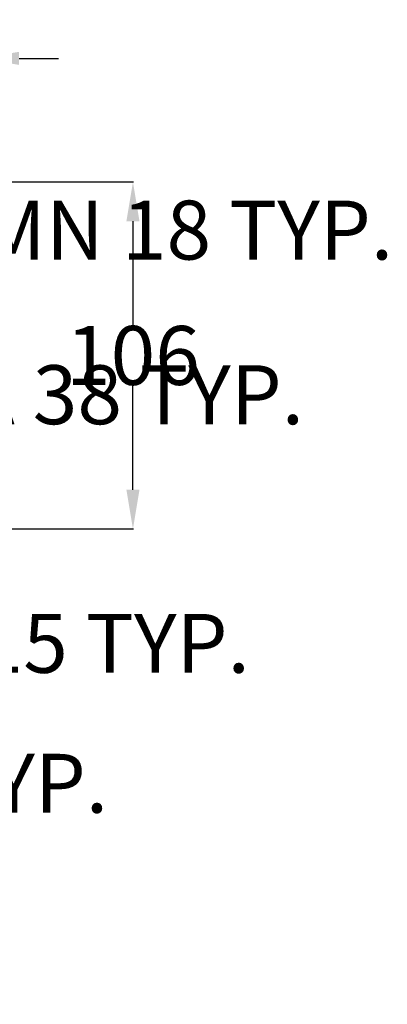
# Model space of a CAD drawing. Units: inches. Extents: x -90 to 536, y -553 to 299.
# Tile 27 of 27: x 410 to 523, y -2 to 299. Entities that reach past the tile are written whole.
import ezdxf

# ---------------------------------------------------------------- set-up
doc = ezdxf.new("R2010")
doc.units = ezdxf.units.IN
doc.layers.add('A-ANNO-DIMS', color=2, linetype='Continuous', lineweight=18)
doc.styles.get("Standard").update_dxf_attribs({"font": 'arial.ttf'})
doc.dimstyles.get("Standard").update_dxf_attribs({"dimtxt": 18, "dimasz": 12, "dimexe": 0.18, "dimexo": 0.0625, "dimgap": 0.09, "dimtad": 0, "dimtih": 1, "dimtoh": 1, "dimdec": 0, "dimzin": 0, "dimdsep": 46, "dimlunit": 3, "dimtxsty": 'Standard', "dimcen": 0.09, "dimadec": 0, "dimazin": 0, "dimtfac": 1, "dimtdec": 0, "dimtofl": 0, "dimtmove": 0, "dimatfit": 3, "dimfxl": 1, "dimtolj": 1, "dimtzin": 0, "dimarcsym": 0})

# ---------------------------------------------------------------- blocks, each defined once
blk = doc.blocks.new('*D19')
at = {"layer": 'A-ANNO-DIMS', "color": 0, "lineweight": -2, "transparency": 16777216}
for p, q in [((299.76, 172.45), (299.76, 184.45)), ((299.76, 184.45), (311.76, 184.45)), ((294.19, 172.45), (299.94, 172.45)), ((299.76, 146.95), (299.76, 160.45)), ((294.19, 134.95), (299.94, 134.95))]:
    blk.add_line(p, q, dxfattribs=at)
at = {"layer": 'A-ANNO-DIMS', "color": 0, "transparency": 16777216}
for points in [[(297.76, 160.45), (301.76, 160.45), (299.76, 172.45)], [(297.76, 146.95), (301.76, 146.95), (299.76, 134.95)]]:
    blk.add_solid(points, dxfattribs=at)
at = {"layer": 'Defpoints', "color": 0, "transparency": 16777216}
for p in [(294.13, 172.45), (299.76, 172.45), (294.13, 134.95)]:
    blk.add_point(p, dxfattribs=at)
at = {"layer": 'A-ANNO-DIMS', "color": 0, "transparency": 16777216, "insert": (408.3, 184.45), "char_height": 18, "attachment_point": 5}
blk.add_mtext('\\A1;DOOR A 38 TYP.', dxfattribs=at)
blk = doc.blocks.new('*D23')
at = {"layer": 'A-ANNO-DIMS', "color": 0, "lineweight": -2, "transparency": 16777216}
for p, q in [((273.13, 234.75), (261.13, 234.75)), ((285.13, 237.38), (285.13, 234.57)), ((303.13, 237.38), (303.13, 234.57)), ((315.13, 234.75), (327.13, 234.75))]:
    blk.add_line(p, q, dxfattribs=at)
at = {"layer": 'A-ANNO-DIMS', "color": 0, "transparency": 16777216}
for points in [[(273.13, 236.75), (273.13, 232.75), (285.13, 234.75)], [(315.13, 236.75), (315.13, 232.75), (303.13, 234.75)]]:
    blk.add_solid(points, dxfattribs=at)
at = {"layer": 'Defpoints', "color": 0, "transparency": 16777216}
for p in [(285.13, 237.45), (303.13, 237.45), (303.13, 234.75)]:
    blk.add_point(p, dxfattribs=at)
at = {"layer": 'A-ANNO-DIMS', "color": 0, "transparency": 16777216, "insert": (428.9, 234.75), "char_height": 18, "attachment_point": 5}
blk.add_mtext('\\A1;COLUMN 18 TYP.', dxfattribs=at)
blk = doc.blocks.new('*D29')
at = {"layer": 'A-ANNO-DIMS', "color": 0, "lineweight": -2, "transparency": 16777216}
for p, q in [((357.07, 98.65), (347.09, 98.65)), ((347.27, 86.65), (347.27, 75.05)), ((347.27, 44.88), (347.27, 56.48)), ((357.07, 32.88), (347.09, 32.88))]:
    blk.add_line(p, q, dxfattribs=at)
at = {"layer": 'A-ANNO-DIMS', "color": 0, "transparency": 16777216}
for points in [[(345.27, 86.65), (349.27, 86.65), (347.27, 98.65)], [(345.27, 44.88), (349.27, 44.88), (347.27, 32.88)]]:
    blk.add_solid(points, dxfattribs=at)
at = {"layer": 'Defpoints', "color": 0, "transparency": 16777216}
for p in [(347.27, 98.65), (357.13, 98.65), (357.13, 32.88)]:
    blk.add_point(p, dxfattribs=at)
at = {"layer": 'A-ANNO-DIMS', "color": 0, "transparency": 16777216, "insert": (347.27, 65.76), "char_height": 18, "attachment_point": 5}
blk.add_mtext('\\A1;TV UNIT 66 TYP.', dxfattribs=at)
blk = doc.blocks.new('*D30')
at = {"layer": 'A-ANNO-DIMS', "color": 0, "lineweight": -2, "transparency": 16777216}
for p, q in [((345.13, 108.51), (333.13, 108.51)), ((357.13, 98.71), (357.13, 108.69)), ((372.13, 98.71), (372.13, 108.69)), ((384.13, 108.51), (396.13, 108.51))]:
    blk.add_line(p, q, dxfattribs=at)
at = {"layer": 'A-ANNO-DIMS', "color": 0, "transparency": 16777216}
for points in [[(345.13, 110.51), (345.13, 106.51), (357.13, 108.51)], [(384.13, 110.51), (384.13, 106.51), (372.13, 108.51)]]:
    blk.add_solid(points, dxfattribs=at)
at = {"layer": 'Defpoints', "color": 0, "transparency": 16777216}
for p in [(372.13, 108.51), (357.13, 98.65), (372.13, 98.65)]:
    blk.add_point(p, dxfattribs=at)
at = {"layer": 'A-ANNO-DIMS', "color": 0, "transparency": 16777216, "insert": (439.18, 108.51), "char_height": 18, "attachment_point": 5}
blk.add_mtext('\\A1;15 TYP.', dxfattribs=at)
blk = doc.blocks.new('*D59')
at = {"layer": 'A-ANNO-DIMS', "color": 0, "lineweight": -2, "transparency": 16777216}
for p, q in [((341.13174, 287.201217), (329.13174, 287.201217)), ((353.13174, -71.491283), (353.13174, 287.381217)), ((398.13174, -71.491283), (398.13174, 287.381217)), ((410.13174, 287.201217), (422.13174, 287.201217))]:
    blk.add_line(p, q, dxfattribs=at)
at = {"layer": 'A-ANNO-DIMS', "color": 0, "transparency": 16777216}
for points in [[(341.13174, 289.201217), (341.13174, 285.201217), (353.13174, 287.201217)], [(410.13174, 289.201217), (410.13174, 285.201217), (398.13174, 287.201217)]]:
    blk.add_solid(points, dxfattribs=at)
at = {"layer": 'Defpoints', "color": 0, "transparency": 16777216}
for p in [(398.13174, 287.201217), (353.13174, -71.553783), (398.13174, -71.553783)]:
    blk.add_point(p, dxfattribs=at)
at = {"layer": 'A-ANNO-DIMS', "color": 0, "transparency": 16777216, "insert": (375.63174, 287.201217), "char_height": 18, "attachment_point": 5}
blk.add_mtext('\\A1;45', dxfattribs=at)
blk = doc.blocks.new('*D66')
at = {"layer": 'A-ANNO-DIMS', "color": 0, "lineweight": -2, "transparency": 16777216}
for p, q in [((303.19, 249.45), (445.07, 249.45)), ((444.89, 237.45), (444.89, 205.73)), ((444.89, 155.45), (444.89, 187.17)), ((381.19, 143.45), (445.07, 143.45))]:
    blk.add_line(p, q, dxfattribs=at)
at = {"layer": 'A-ANNO-DIMS', "color": 0, "transparency": 16777216}
for points in [[(442.89, 237.45), (446.89, 237.45), (444.89, 249.45)], [(442.89, 155.45), (446.89, 155.45), (444.89, 143.45)]]:
    blk.add_solid(points, dxfattribs=at)
at = {"layer": 'Defpoints', "color": 0, "transparency": 16777216}
for p in [(303.13, 249.45), (444.89, 249.45), (381.13, 143.45)]:
    blk.add_point(p, dxfattribs=at)
at = {"layer": 'A-ANNO-DIMS', "color": 0, "transparency": 16777216, "insert": (444.89, 196.45), "char_height": 18, "attachment_point": 5}
blk.add_mtext('\\A1;106', dxfattribs=at)

msp = doc.modelspace()

# ---------------------------------------------------------------- dimensions: what is measured, and where the dimension line sits
at = {"layer": 'A-ANNO-DIMS'}
dim = msp.add_linear_dim(base=(398.1317, 287.2012), p1=(353.1317, -71.5538), p2=(398.1317, -71.5538), dimstyle='Standard', override={"dimdec": 0, "dimlfac": 1, "dimrnd": 0, "dimzin": 0, "dimdsep": 46, "dimlunit": 2}, dxfattribs=at)
dim.commit()
dim.dimension.update_dxf_attribs({"geometry": '*D59', "text_midpoint": (375.6317, 287.2012)})
for base, p1, p2, angle, text, picture, middle in [((303.1317, 234.7462), (285.1317, 237.4462), (303.1317, 237.4462), 0, 'COLUMN <> TYP.', '*D23', (428.9046, 234.7462)), ((299.7567404714, 172.4462174295), (294.1317404714, 134.9462174295), (294.1317404714, 172.4462174295), 90, 'DOOR A <> TYP.', '*D19', (408.2989914946, 184.4462174295)), ((347.2664, 98.6495), (357.1317, 32.8805), (357.1317, 98.6495), 90, 'TV UNIT <> TYP.', '*D29', (347.2664, 65.765))]:
    dim = msp.add_linear_dim(base=base, p1=p1, p2=p2, angle=angle, text=text, dimstyle='Standard', override={"dimdec": 0, "dimlfac": 1, "dimrnd": 0, "dimzin": 0, "dimdsep": 46, "dimlunit": 2}, dxfattribs=at)
    dim.commit()
    dim.dimension.update_dxf_attribs({"geometry": picture, "text_midpoint": middle})
dim = msp.add_linear_dim(base=(444.8867, 249.4462), p1=(381.1317, 143.4462), p2=(303.1317, 249.4462), angle=90, dimstyle='Standard', override={"dimdec": 0, "dimlfac": 1, "dimrnd": 0, "dimzin": 0, "dimdsep": 46, "dimlunit": 2}, dxfattribs=at)
dim.commit()
dim.dimension.update_dxf_attribs({"geometry": '*D66', "text_midpoint": (444.8867, 196.4462)})
dim = msp.add_linear_dim(base=(372.1317, 108.5148), p1=(357.1317, 98.6495), p2=(372.1317, 98.6495), text='<> TYP.', dimstyle='Standard', override={"dimdec": 0, "dimlfac": 1, "dimrnd": 0, "dimzin": 0, "dimdsep": 46, "dimlunit": 2}, dxfattribs=at)
dim.commit()
dim.dimension.update_dxf_attribs({"geometry": '*D30', "text_midpoint": (439.1835, 108.5148)})

doc.saveas('drawing.dxf')
